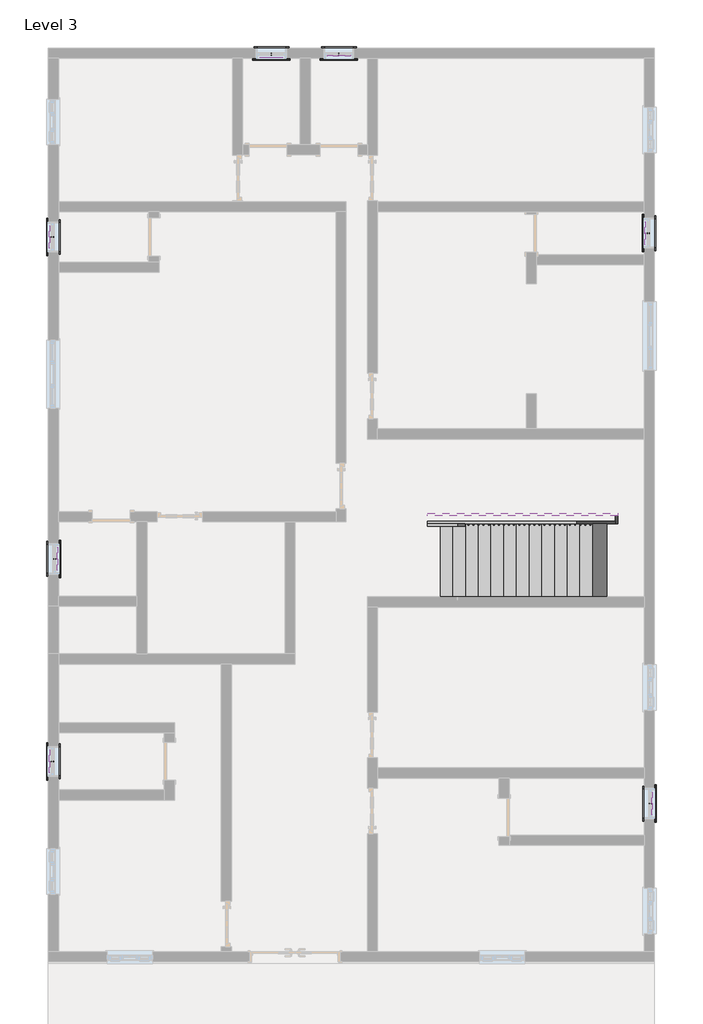
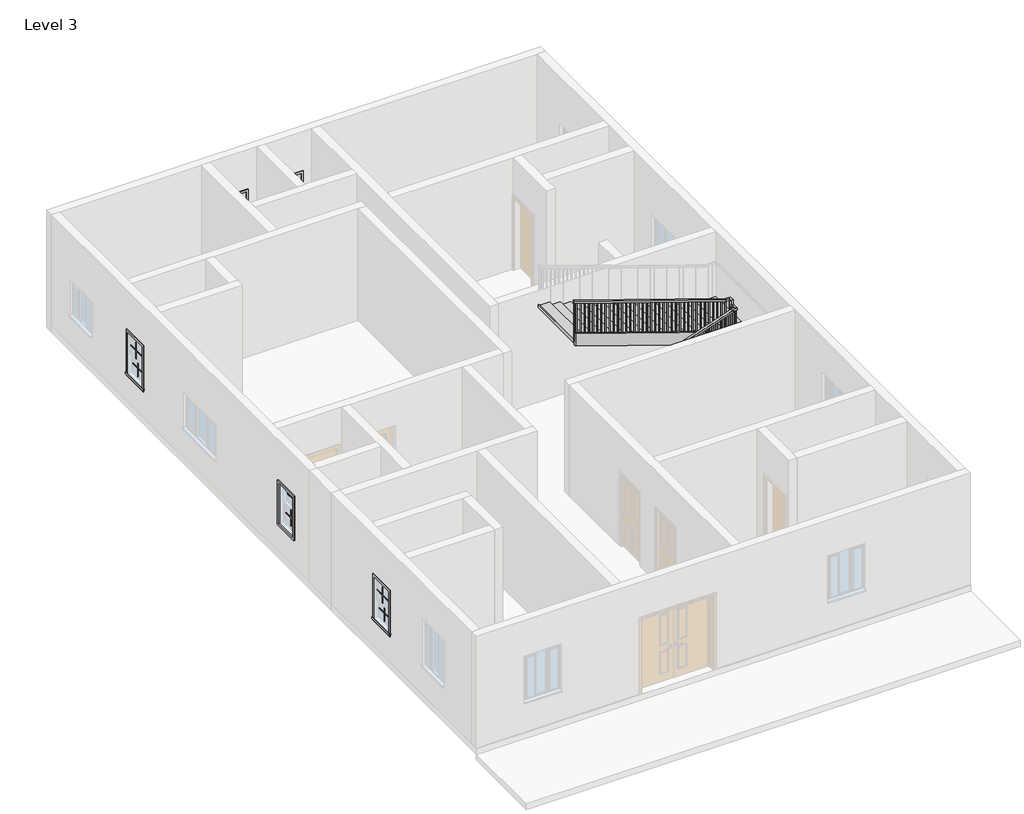
# One storey, part 3 of 3: 28 proxies, 6 members, 1 railing, 1 stair flight.
"""IFC4 building model written with IfcOpenShell, lengths in millimetres."""

from ifc_helpers import new_model, si_unit, frame, origin, place, context, project, spatial, polyline, outline, extrude, faceted_brep, transform, mapped, element, save
from components import muntin_pattern_2x2_muntin_pattern_2x2_eba6c5fb, trim_window_exterior_flat_with_sill_278e6a94, trim_window_interior_flat_picture_frame_e9fd5f45, stair_flight_242bbcd4

model = new_model("IFC4")

# Units and contexts
model_context = context("Model", 3, world=origin())
ifc_project = project(units=[si_unit("LENGTHUNIT", "METRE", prefix="MILLI")], contexts=[model_context])

# Site, building, storey
site = spatial("IfcSite", under=ifc_project)
building = spatial("IfcBuilding", under=site)
storey = spatial("IfcBuildingStorey", under=building, Name="Level 3", Elevation=6096.0)

# Proxies
placement = place(None, origin())
muntin_pattern_2x2_muntin_pattern_2x2_shape = muntin_pattern_2x2_muntin_pattern_2x2_eba6c5fb(model_context)
element("IfcBuildingElementProxy", 1, Name="Muntin Pattern_2x2 : Muntin Pattern_2x2", ObjectType="Muntin Pattern_2x2 : Muntin Pattern_2x2", at=placement, inside=storey, context=model_context, shape_type="MappedRepresentation", body=[
    mapped(muntin_pattern_2x2_muntin_pattern_2x2_shape, transform((-6096.8589448, 5183.1303322, 7566.025), x_axis=(0.0, 1.0, 0.0), y_axis=(-1.0, 0.0, 0.0), z_axis=(0.0, 0.0, 1.0))),
])
element("IfcBuildingElementProxy", 2, Name="Muntin Pattern_2x2 : Muntin Pattern_2x2", ObjectType="Muntin Pattern_2x2 : Muntin Pattern_2x2", at=placement, inside=storey, context=model_context, shape_type="MappedRepresentation", body=[
    mapped(muntin_pattern_2x2_muntin_pattern_2x2_shape, transform((-6052.4089448, 5183.1303322, 7086.6), x_axis=(0.0, 1.0, 0.0), y_axis=(-1.0, 0.0, 0.0), z_axis=(0.0, 0.0, 1.0))),
])
element("IfcBuildingElementProxy", 3, Name="Muntin Pattern_2x2 : Muntin Pattern_2x2", ObjectType="Muntin Pattern_2x2 : Muntin Pattern_2x2", at=placement, inside=storey, context=model_context, shape_type="MappedRepresentation", body=[
    mapped(muntin_pattern_2x2_muntin_pattern_2x2_shape, transform((-1673.5309118, 8787.5224079, 7566.025), x_axis=(-1.0, 0.0, 0.0), y_axis=(0.0, -1.0, 0.0), z_axis=(0.0, 0.0, 1.0))),
])
element("IfcBuildingElementProxy", 4, Name="Muntin Pattern_2x2 : Muntin Pattern_2x2", ObjectType="Muntin Pattern_2x2 : Muntin Pattern_2x2", at=placement, inside=storey, context=model_context, shape_type="MappedRepresentation", body=[
    mapped(muntin_pattern_2x2_muntin_pattern_2x2_shape, transform((-1673.5309118, 8831.9724079, 7086.6), x_axis=(-1.0, 0.0, 0.0), y_axis=(0.0, -1.0, 0.0), z_axis=(0.0, 0.0, 1.0))),
])
element("IfcBuildingElementProxy", 5, Name="Muntin Pattern_2x2 : Muntin Pattern_2x2", ObjectType="Muntin Pattern_2x2 : Muntin Pattern_2x2", at=placement, inside=storey, context=model_context, shape_type="MappedRepresentation", body=[
    mapped(muntin_pattern_2x2_muntin_pattern_2x2_shape, transform((-324.5451949, 8787.5224079, 7566.025), x_axis=(-1.0, 0.0, 0.0), y_axis=(0.0, -1.0, 0.0), z_axis=(0.0, 0.0, 1.0))),
])
element("IfcBuildingElementProxy", 6, Name="Muntin Pattern_2x2 : Muntin Pattern_2x2", ObjectType="Muntin Pattern_2x2 : Muntin Pattern_2x2", at=placement, inside=storey, context=model_context, shape_type="MappedRepresentation", body=[
    mapped(muntin_pattern_2x2_muntin_pattern_2x2_shape, transform((-324.5451949, 8831.9724079, 7086.6), x_axis=(-1.0, 0.0, 0.0), y_axis=(0.0, -1.0, 0.0), z_axis=(0.0, 0.0, 1.0))),
])
element("IfcBuildingElementProxy", 7, Name="Muntin Pattern_2x2 : Muntin Pattern_2x2", ObjectType="Muntin Pattern_2x2 : Muntin Pattern_2x2", at=placement, inside=storey, context=model_context, shape_type="MappedRepresentation", body=[
    mapped(muntin_pattern_2x2_muntin_pattern_2x2_shape, transform((5813.4689795, 5259.3303322, 7566.025), x_axis=(0.0, 1.0, 0.0), y_axis=(-1.0, 0.0, 0.0), z_axis=(0.0, 0.0, 1.0))),
])
element("IfcBuildingElementProxy", 8, Name="Muntin Pattern_2x2 : Muntin Pattern_2x2", ObjectType="Muntin Pattern_2x2 : Muntin Pattern_2x2", at=placement, inside=storey, context=model_context, shape_type="MappedRepresentation", body=[
    mapped(muntin_pattern_2x2_muntin_pattern_2x2_shape, transform((5857.9189795, 5259.3303322, 7086.6), x_axis=(0.0, 1.0, 0.0), y_axis=(-1.0, 0.0, 0.0), z_axis=(0.0, 0.0, 1.0))),
])
element("IfcBuildingElementProxy", 9, Name="Muntin Pattern_2x2 : Muntin Pattern_2x2", ObjectType="Muntin Pattern_2x2 : Muntin Pattern_2x2", at=placement, inside=storey, context=model_context, shape_type="MappedRepresentation", body=[
    mapped(muntin_pattern_2x2_muntin_pattern_2x2_shape, transform((5946.8189795, -6133.2488489, 7566.025), x_axis=(0.0, -1.0, 0.0), y_axis=(1.0, 0.0, 0.0), z_axis=(0.0, 0.0, 1.0))),
])
element("IfcBuildingElementProxy", 10, Name="Muntin Pattern_2x2 : Muntin Pattern_2x2", ObjectType="Muntin Pattern_2x2 : Muntin Pattern_2x2", at=placement, inside=storey, context=model_context, shape_type="MappedRepresentation", body=[
    mapped(muntin_pattern_2x2_muntin_pattern_2x2_shape, transform((5902.3689795, -6133.2488489, 7086.6), x_axis=(0.0, -1.0, 0.0), y_axis=(1.0, 0.0, 0.0), z_axis=(0.0, 0.0, 1.0))),
])
element("IfcBuildingElementProxy", 11, Name="Muntin Pattern_2x2 : Muntin Pattern_2x2", ObjectType="Muntin Pattern_2x2 : Muntin Pattern_2x2", at=placement, inside=storey, context=model_context, shape_type="MappedRepresentation", body=[
    mapped(muntin_pattern_2x2_muntin_pattern_2x2_shape, transform((-6096.8589448, -5291.0659014, 7566.025), x_axis=(0.0, 1.0, 0.0), y_axis=(-1.0, 0.0, 0.0), z_axis=(0.0, 0.0, 1.0))),
])
element("IfcBuildingElementProxy", 12, Name="Muntin Pattern_2x2 : Muntin Pattern_2x2", ObjectType="Muntin Pattern_2x2 : Muntin Pattern_2x2", at=placement, inside=storey, context=model_context, shape_type="MappedRepresentation", body=[
    mapped(muntin_pattern_2x2_muntin_pattern_2x2_shape, transform((-6052.4089448, -5291.0659014, 7086.6), x_axis=(0.0, 1.0, 0.0), y_axis=(-1.0, 0.0, 0.0), z_axis=(0.0, 0.0, 1.0))),
])
element("IfcBuildingElementProxy", 13, Name="Muntin Pattern_2x2 : Muntin Pattern_2x2", ObjectType="Muntin Pattern_2x2 : Muntin Pattern_2x2", at=placement, inside=storey, context=model_context, shape_type="MappedRepresentation", body=[
    mapped(muntin_pattern_2x2_muntin_pattern_2x2_shape, transform((-5963.5089448, -1246.1159014, 7566.025), x_axis=(0.0, -1.0, 0.0), y_axis=(1.0, 0.0, 0.0), z_axis=(0.0, 0.0, 1.0))),
])
element("IfcBuildingElementProxy", 14, Name="Muntin Pattern_2x2 : Muntin Pattern_2x2", ObjectType="Muntin Pattern_2x2 : Muntin Pattern_2x2", at=placement, inside=storey, context=model_context, shape_type="MappedRepresentation", body=[
    mapped(muntin_pattern_2x2_muntin_pattern_2x2_shape, transform((-6007.9589448, -1246.1159014, 7086.6), x_axis=(0.0, -1.0, 0.0), y_axis=(1.0, 0.0, 0.0), z_axis=(0.0, 0.0, 1.0))),
])
trim_window_exterior_flat_with_sill_shape = trim_window_exterior_flat_with_sill_278e6a94(model_context)
element("IfcBuildingElementProxy", 15, Name="Trim-Window-Exterior-Flat : with Sill", ObjectType="Trim-Window-Exterior-Flat : with Sill", at=placement, inside=storey, context=model_context, shape_type="MappedRepresentation", body=[
    mapped(trim_window_exterior_flat_with_sill_shape, transform((-6131.7839448, 5183.1303322, 8077.2), x_axis=(0.0, -1.0, 0.0), y_axis=(0.0, 0.0, 1.0), z_axis=(-1.0, 0.0, 0.0))),
])
element("IfcBuildingElementProxy", 16, Name="Trim-Window-Exterior-Flat : with Sill", ObjectType="Trim-Window-Exterior-Flat : with Sill", at=placement, inside=storey, context=model_context, shape_type="MappedRepresentation", body=[
    mapped(trim_window_exterior_flat_with_sill_shape, transform((-1673.5309118, 8752.5974079, 8077.2), x_axis=(1.0, 0.0, 0.0), y_axis=(0.0, 0.0, 1.0), z_axis=(0.0, -1.0, 0.0))),
])
element("IfcBuildingElementProxy", 17, Name="Trim-Window-Exterior-Flat : with Sill", ObjectType="Trim-Window-Exterior-Flat : with Sill", at=placement, inside=storey, context=model_context, shape_type="MappedRepresentation", body=[
    mapped(trim_window_exterior_flat_with_sill_shape, transform((-324.5451949, 8752.5974079, 8077.2), x_axis=(1.0, 0.0, 0.0), y_axis=(0.0, 0.0, 1.0), z_axis=(0.0, -1.0, 0.0))),
])
element("IfcBuildingElementProxy", 18, Name="Trim-Window-Exterior-Flat : with Sill", ObjectType="Trim-Window-Exterior-Flat : with Sill", at=placement, inside=storey, context=model_context, shape_type="MappedRepresentation", body=[
    mapped(trim_window_exterior_flat_with_sill_shape, transform((5778.5439795, 5259.3303322, 8077.2), x_axis=(0.0, -1.0, 0.0), y_axis=(0.0, 0.0, 1.0), z_axis=(-1.0, 0.0, 0.0))),
])
element("IfcBuildingElementProxy", 19, Name="Trim-Window-Exterior-Flat : with Sill", ObjectType="Trim-Window-Exterior-Flat : with Sill", at=placement, inside=storey, context=model_context, shape_type="MappedRepresentation", body=[
    mapped(trim_window_exterior_flat_with_sill_shape, transform((5981.7439795, -6133.2488489, 8077.2), x_axis=(0.0, 1.0, 0.0), y_axis=(0.0, 0.0, 1.0), z_axis=(1.0, 0.0, 0.0))),
])
element("IfcBuildingElementProxy", 20, Name="Trim-Window-Exterior-Flat : with Sill", ObjectType="Trim-Window-Exterior-Flat : with Sill", at=placement, inside=storey, context=model_context, shape_type="MappedRepresentation", body=[
    mapped(trim_window_exterior_flat_with_sill_shape, transform((-6131.7839448, -5291.0659014, 8077.2), x_axis=(0.0, -1.0, 0.0), y_axis=(0.0, 0.0, 1.0), z_axis=(-1.0, 0.0, 0.0))),
])
element("IfcBuildingElementProxy", 21, Name="Trim-Window-Exterior-Flat : with Sill", ObjectType="Trim-Window-Exterior-Flat : with Sill", at=placement, inside=storey, context=model_context, shape_type="MappedRepresentation", body=[
    mapped(trim_window_exterior_flat_with_sill_shape, transform((-5928.5839448, -1246.1159014, 8077.2), x_axis=(0.0, 1.0, 0.0), y_axis=(0.0, 0.0, 1.0), z_axis=(1.0, 0.0, 0.0))),
])
trim_window_interior_flat_picture_frame_shape = trim_window_interior_flat_picture_frame_e9fd5f45(model_context)
element("IfcBuildingElementProxy", 22, Name="Trim-Window-Interior-Flat : Picture Frame", ObjectType="Trim-Window-Interior-Flat : Picture Frame", at=placement, inside=storey, context=model_context, shape_type="MappedRepresentation", body=[
    mapped(trim_window_interior_flat_picture_frame_shape, transform((-5928.5839448, 5183.1303322, 8077.2), x_axis=(0.0, 1.0, 0.0), y_axis=(0.0, 0.0, 1.0), z_axis=(1.0, 0.0, 0.0))),
])
element("IfcBuildingElementProxy", 23, Name="Trim-Window-Interior-Flat : Picture Frame", ObjectType="Trim-Window-Interior-Flat : Picture Frame", at=placement, inside=storey, context=model_context, shape_type="MappedRepresentation", body=[
    mapped(trim_window_interior_flat_picture_frame_shape, transform((-1673.5309118, 8955.7974079, 8077.2), x_axis=(-1.0, 0.0, 0.0), y_axis=(0.0, 0.0, 1.0), z_axis=(0.0, 1.0, 0.0))),
])
element("IfcBuildingElementProxy", 24, Name="Trim-Window-Interior-Flat : Picture Frame", ObjectType="Trim-Window-Interior-Flat : Picture Frame", at=placement, inside=storey, context=model_context, shape_type="MappedRepresentation", body=[
    mapped(trim_window_interior_flat_picture_frame_shape, transform((-324.5451949, 8955.7974079, 8077.2), x_axis=(-1.0, 0.0, 0.0), y_axis=(0.0, 0.0, 1.0), z_axis=(0.0, 1.0, 0.0))),
])
element("IfcBuildingElementProxy", 25, Name="Trim-Window-Interior-Flat : Picture Frame", ObjectType="Trim-Window-Interior-Flat : Picture Frame", at=placement, inside=storey, context=model_context, shape_type="MappedRepresentation", body=[
    mapped(trim_window_interior_flat_picture_frame_shape, transform((5981.7439795, 5259.3303322, 8077.2), x_axis=(0.0, 1.0, 0.0), y_axis=(0.0, 0.0, 1.0), z_axis=(1.0, 0.0, 0.0))),
])
element("IfcBuildingElementProxy", 26, Name="Trim-Window-Interior-Flat : Picture Frame", ObjectType="Trim-Window-Interior-Flat : Picture Frame", at=placement, inside=storey, context=model_context, shape_type="MappedRepresentation", body=[
    mapped(trim_window_interior_flat_picture_frame_shape, transform((5778.5439795, -6133.2488489, 8077.2), x_axis=(0.0, -1.0, 0.0), y_axis=(0.0, 0.0, 1.0), z_axis=(-1.0, 0.0, 0.0))),
])
element("IfcBuildingElementProxy", 27, Name="Trim-Window-Interior-Flat : Picture Frame", ObjectType="Trim-Window-Interior-Flat : Picture Frame", at=placement, inside=storey, context=model_context, shape_type="MappedRepresentation", body=[
    mapped(trim_window_interior_flat_picture_frame_shape, transform((-5928.5839448, -5291.0659014, 8077.2), x_axis=(0.0, 1.0, 0.0), y_axis=(0.0, 0.0, 1.0), z_axis=(1.0, 0.0, 0.0))),
])
element("IfcBuildingElementProxy", 28, Name="Trim-Window-Interior-Flat : Picture Frame", ObjectType="Trim-Window-Interior-Flat : Picture Frame", at=placement, inside=storey, context=model_context, shape_type="MappedRepresentation", body=[
    mapped(trim_window_interior_flat_picture_frame_shape, transform((-6131.7839448, -1246.1159014, 8077.2), x_axis=(0.0, -1.0, 0.0), y_axis=(0.0, 0.0, 1.0), z_axis=(-1.0, 0.0, 0.0))),
])

# Members
element("IfcMember", 29, ObjectType="Stringer - 2\" Width", at=placement, inside=storey, context=model_context, shape_type="SweptSolid", body=[
    extrude(outline(polyline([(6289.7751932, 1449.3932247), (6096.0, 1449.3932247), (6096.0, 1827.5890963), (7236.094539, 5195.8669505), (7543.8, 5195.8669505), (7543.8, 5154.2649181), (6289.7751932, 1449.3932247)])), frame((0.0, -541.2659014, 0.0), z_axis=(0.0, 1.0, 0.0), x_axis=(0.0, 0.0, 1.0)), (0.0, 0.0, 1.0), 50.8),
])
element("IfcMember", 30, ObjectType="Stringer - 2\" Width", at=placement, inside=storey, context=model_context, shape_type="SweptSolid", body=[
    extrude(outline(polyline([(5246.6669505, -541.2659014), (5195.8669505, -541.2659014), (5195.8669505, -388.7910016), (5246.6669505, -388.7910016), (5246.6669505, -541.2659014)])), frame((0.0, 0.0, 7239.0), z_axis=(0.0, 0.0, 1.0), x_axis=(1.0, 0.0, 0.0)), (0.0, 0.0, 1.0), 304.8),
])
element("IfcMember", 31, ObjectType="Stringer - 2\" Width", at=placement, inside=storey, context=model_context, shape_type="SweptSolid", body=[
    extrude(outline(polyline([(7339.0143208, 5246.6669505), (7660.8012358, 5246.6669505), (8946.1022784, 1449.3932247), (8624.3153634, 1449.3932247), (7339.0143208, 5246.6669505)])), frame((0.0, -388.7910016, 0.0), z_axis=(0.0, 1.0, 0.0), x_axis=(0.0, 0.0, 1.0)), (0.0, 0.0, 1.0), 50.8),
])
element("IfcMember", 32, ObjectType="Stringer - 2\" Width", at=placement, inside=storey, context=model_context, shape_type="SweptSolid", body=[
    extrude(outline(polyline([(6289.7751932, 1449.3932247), (6096.0, 1449.3932247), (6096.0, 1827.5890963), (7448.1142723, 5822.2548051), (7543.8, 5822.2548051), (7543.8, 5154.2649181), (6289.7751932, 1449.3932247)])), frame((0.0, -2116.0659014, 0.0), z_axis=(0.0, 1.0, 0.0), x_axis=(0.0, 0.0, 1.0)), (0.0, 0.0, 1.0), 50.8),
])
element("IfcMember", 33, ObjectType="Stringer - 2\" Width", at=placement, inside=storey, context=model_context, shape_type="SweptSolid", body=[
    extrude(outline(polyline([(5873.0548051, -2116.0659014), (5822.2548051, -2116.0659014), (5822.2548051, 1185.9340986), (5873.0548051, 1185.9340986), (5873.0548051, -2116.0659014)])), frame((0.0, 0.0, 7239.0), z_axis=(0.0, 0.0, 1.0), x_axis=(1.0, 0.0, 0.0)), (0.0, 0.0, 1.0), 304.8),
])
element("IfcMember", 34, ObjectType="Stringer - 2\" Width", at=placement, inside=storey, context=model_context, shape_type="SweptSolid", body=[
    extrude(outline(polyline([(7239.0, 5873.0548051), (7448.7815025, 5873.0548051), (8946.1022784, 1449.3932247), (8624.3153634, 1449.3932247), (7239.0, 5542.1477288), (7239.0, 5873.0548051)])), frame((0.0, 1185.9340986, 0.0), z_axis=(0.0, 1.0, 0.0), x_axis=(0.0, 0.0, 1.0)), (0.0, 0.0, 1.0), 50.8),
])

# Railing
element("IfcRailing", 35, ObjectType="Handrail - Rectangular", at=placement, inside=storey, context=model_context, shape_type="SolidModel", body=[
    faceted_brep([(1449.3932247, -541.2659014, 7096.125), (1449.3932247, -541.2659014, 7042.4913852), (1449.3932247, -592.0659014, 7042.4913852), (1449.3932247, -592.0659014, 7096.125), (5170.4669505, -541.2659014, 8356.1963098), (5221.2669505, -541.2659014, 8319.7651551), (5221.2669505, -592.0659014, 8319.7651551), (5170.4669505, -592.0659014, 8356.1963098), (5170.4669505, -541.2659014, 8382.0), (5221.2669505, -541.2659014, 8331.2), (5221.2669505, -592.0659014, 8331.2), (5170.4669505, -592.0659014, 8382.0), (5246.6669505, -541.2659014, 8382.0), (5246.6669505, -541.2659014, 8331.2), (5297.4669505, -592.0659014, 8331.2), (5297.4669505, -592.0659014, 8382.0), (5246.6669505, -465.0659014, 8382.0), (5246.6669505, -465.0659014, 8331.2), (5297.4669505, -465.0659014, 8331.2), (5297.4669505, -465.0659014, 8382.0), (5246.6669505, -414.1910016, 8382.0), (5246.6669505, -363.3910016, 8331.2), (5297.4669505, -363.3910016, 8331.2), (5297.4669505, -414.1910016, 8382.0), (5246.6669505, -414.1910016, 8493.5286902), (5246.6669505, -363.3910016, 8442.7286902), (5297.4669505, -363.3910016, 8442.7286902), (5297.4669505, -414.1910016, 8493.5286902), (5246.6669505, -337.9910016, 8493.5286902), (5246.6669505, -337.9910016, 8442.7286902), (5297.4669505, -287.1910016, 8442.7286902), (5297.4669505, -287.1910016, 8493.5286902), (5170.4669505, -337.9910016, 8493.5286902), (5162.099099, -337.9910016, 8442.7286902), (5162.099099, -287.1910016, 8442.7286902), (5170.4669505, -287.1910016, 8493.5286902), (1449.3932247, -337.9910016, 9753.6), (1449.3932247, -287.1910016, 9753.6), (1449.3932247, -287.1910016, 9699.9663852), (1449.3932247, -337.9910016, 9699.9663852)], [[[0, 1, 2, 3]], [[1, 0, 4, 5]], [[2, 1, 5, 6]], [[3, 2, 6, 7]], [[0, 3, 7, 4]], [[5, 4, 8, 9]], [[6, 5, 9, 10]], [[7, 6, 10, 11]], [[4, 7, 11, 8]], [[9, 8, 12, 13]], [[10, 9, 13, 14]], [[11, 10, 14, 15]], [[8, 11, 15, 12]], [[13, 12, 16, 17]], [[14, 13, 17, 18]], [[15, 14, 18, 19]], [[12, 15, 19, 16]], [[17, 16, 20, 21]], [[18, 17, 21, 22]], [[19, 18, 22, 23]], [[16, 19, 23, 20]], [[21, 20, 24, 25]], [[22, 21, 25, 26]], [[23, 22, 26, 27]], [[20, 23, 27, 24]], [[25, 24, 28, 29]], [[26, 25, 29, 30]], [[27, 26, 30, 31]], [[24, 27, 31, 28]], [[29, 28, 32, 33]], [[30, 29, 33, 34]], [[31, 30, 34, 35]], [[28, 31, 35, 32]], [[36, 37, 38, 39]], [[33, 32, 36, 39]], [[34, 33, 39, 38]], [[35, 34, 38, 37]], [[32, 35, 37, 36]]]),
    extrude(outline(polyline([(9681.6976686, 1503.3419505), (8753.475, 1503.3419505), (8753.475, 1522.3919505), (9675.246746, 1522.3919505), (9681.6976686, 1503.3419505)])), frame((0.0, -322.1160016, 0.0), z_axis=(0.0, 1.0, 0.0), x_axis=(0.0, 0.0, 1.0)), (0.0, 0.0, 1.0), 19.05),
    extrude(outline(polyline([(9647.2927482, 1604.9419505), (8753.475, 1604.9419505), (8753.475, 1623.9919505), (9640.8418257, 1623.9919505), (9647.2927482, 1604.9419505)])), frame((0.0, -322.1160016, 0.0), z_axis=(0.0, 1.0, 0.0), x_axis=(0.0, 0.0, 1.0)), (0.0, 0.0, 1.0), 19.05),
    extrude(outline(polyline([(9612.8878279, 1706.5419505), (8667.75, 1706.5419505), (8667.75, 1725.5919505), (9606.4369054, 1725.5919505), (9612.8878279, 1706.5419505)])), frame((0.0, -322.1160016, 0.0), z_axis=(0.0, 1.0, 0.0), x_axis=(0.0, 0.0, 1.0)), (0.0, 0.0, 1.0), 19.05),
    extrude(outline(polyline([(9578.4829076, 1808.1419505), (8667.75, 1808.1419505), (8667.75, 1827.1919505), (9572.031985, 1827.1919505), (9578.4829076, 1808.1419505)])), frame((0.0, -322.1160016, 0.0), z_axis=(0.0, 1.0, 0.0), x_axis=(0.0, 0.0, 1.0)), (0.0, 0.0, 1.0), 19.05),
    extrude(outline(polyline([(9544.0779873, 1909.7419505), (8667.75, 1909.7419505), (8667.75, 1928.7919505), (9537.6270647, 1928.7919505), (9544.0779873, 1909.7419505)])), frame((0.0, -322.1160016, 0.0), z_axis=(0.0, 1.0, 0.0), x_axis=(0.0, 0.0, 1.0)), (0.0, 0.0, 1.0), 19.05),
    extrude(outline(polyline([(9509.6730669, 2011.3419505), (8582.025, 2011.3419505), (8582.025, 2030.3919505), (9503.2221444, 2030.3919505), (9509.6730669, 2011.3419505)])), frame((0.0, -322.1160016, 0.0), z_axis=(0.0, 1.0, 0.0), x_axis=(0.0, 0.0, 1.0)), (0.0, 0.0, 1.0), 19.05),
    extrude(outline(polyline([(9475.2681466, 2112.9419505), (8582.025, 2112.9419505), (8582.025, 2131.9919505), (9468.817224, 2131.9919505), (9475.2681466, 2112.9419505)])), frame((0.0, -322.1160016, 0.0), z_axis=(0.0, 1.0, 0.0), x_axis=(0.0, 0.0, 1.0)), (0.0, 0.0, 1.0), 19.05),
    extrude(outline(polyline([(9440.8632263, 2214.5419505), (8496.3, 2214.5419505), (8496.3, 2233.5919505), (9434.4123037, 2233.5919505), (9440.8632263, 2214.5419505)])), frame((0.0, -322.1160016, 0.0), z_axis=(0.0, 1.0, 0.0), x_axis=(0.0, 0.0, 1.0)), (0.0, 0.0, 1.0), 19.05),
    extrude(outline(polyline([(9406.4583059, 2316.1419505), (8496.3, 2316.1419505), (8496.3, 2335.1919505), (9400.0073834, 2335.1919505), (9406.4583059, 2316.1419505)])), frame((0.0, -322.1160016, 0.0), z_axis=(0.0, 1.0, 0.0), x_axis=(0.0, 0.0, 1.0)), (0.0, 0.0, 1.0), 19.05),
    extrude(outline(polyline([(9372.0533856, 2417.7419505), (8496.3, 2417.7419505), (8496.3, 2436.7919505), (9365.6024631, 2436.7919505), (9372.0533856, 2417.7419505)])), frame((0.0, -322.1160016, 0.0), z_axis=(0.0, 1.0, 0.0), x_axis=(0.0, 0.0, 1.0)), (0.0, 0.0, 1.0), 19.05),
    extrude(outline(polyline([(9337.6484653, 2519.3419505), (8410.575, 2519.3419505), (8410.575, 2538.3919505), (9331.1975427, 2538.3919505), (9337.6484653, 2519.3419505)])), frame((0.0, -322.1160016, 0.0), z_axis=(0.0, 1.0, 0.0), x_axis=(0.0, 0.0, 1.0)), (0.0, 0.0, 1.0), 19.05),
    extrude(outline(polyline([(9303.243545, 2620.9419505), (8410.575, 2620.9419505), (8410.575, 2639.9919505), (9296.7926224, 2639.9919505), (9303.243545, 2620.9419505)])), frame((0.0, -322.1160016, 0.0), z_axis=(0.0, 1.0, 0.0), x_axis=(0.0, 0.0, 1.0)), (0.0, 0.0, 1.0), 19.05),
    extrude(outline(polyline([(9268.8386246, 2722.5419505), (8324.85, 2722.5419505), (8324.85, 2741.5919505), (9262.3877021, 2741.5919505), (9268.8386246, 2722.5419505)])), frame((0.0, -322.1160016, 0.0), z_axis=(0.0, 1.0, 0.0), x_axis=(0.0, 0.0, 1.0)), (0.0, 0.0, 1.0), 19.05),
    extrude(outline(polyline([(9234.4337043, 2824.1419505), (8324.85, 2824.1419505), (8324.85, 2843.1919505), (9227.9827817, 2843.1919505), (9234.4337043, 2824.1419505)])), frame((0.0, -322.1160016, 0.0), z_axis=(0.0, 1.0, 0.0), x_axis=(0.0, 0.0, 1.0)), (0.0, 0.0, 1.0), 19.05),
    extrude(outline(polyline([(9200.028784, 2925.7419505), (8324.85, 2925.7419505), (8324.85, 2944.7919505), (9193.5778614, 2944.7919505), (9200.028784, 2925.7419505)])), frame((0.0, -322.1160016, 0.0), z_axis=(0.0, 1.0, 0.0), x_axis=(0.0, 0.0, 1.0)), (0.0, 0.0, 1.0), 19.05),
    extrude(outline(polyline([(9165.6238636, 3027.3419505), (8239.125, 3027.3419505), (8239.125, 3046.3919505), (9159.1729411, 3046.3919505), (9165.6238636, 3027.3419505)])), frame((0.0, -322.1160016, 0.0), z_axis=(0.0, 1.0, 0.0), x_axis=(0.0, 0.0, 1.0)), (0.0, 0.0, 1.0), 19.05),
    extrude(outline(polyline([(9131.2189433, 3128.9419505), (8239.125, 3128.9419505), (8239.125, 3147.9919505), (9124.7680208, 3147.9919505), (9131.2189433, 3128.9419505)])), frame((0.0, -322.1160016, 0.0), z_axis=(0.0, 1.0, 0.0), x_axis=(0.0, 0.0, 1.0)), (0.0, 0.0, 1.0), 19.05),
    extrude(outline(polyline([(9096.814023, 3230.5419505), (8153.4, 3230.5419505), (8153.4, 3249.5919505), (9090.3631004, 3249.5919505), (9096.814023, 3230.5419505)])), frame((0.0, -322.1160016, 0.0), z_axis=(0.0, 1.0, 0.0), x_axis=(0.0, 0.0, 1.0)), (0.0, 0.0, 1.0), 19.05),
    extrude(outline(polyline([(9062.4091027, 3332.1419505), (8153.4, 3332.1419505), (8153.4, 3351.1919505), (9055.9581801, 3351.1919505), (9062.4091027, 3332.1419505)])), frame((0.0, -322.1160016, 0.0), z_axis=(0.0, 1.0, 0.0), x_axis=(0.0, 0.0, 1.0)), (0.0, 0.0, 1.0), 19.05),
    extrude(outline(polyline([(9028.0041823, 3433.7419505), (8153.4, 3433.7419505), (8153.4, 3452.7919505), (9021.5532598, 3452.7919505), (9028.0041823, 3433.7419505)])), frame((0.0, -322.1160016, 0.0), z_axis=(0.0, 1.0, 0.0), x_axis=(0.0, 0.0, 1.0)), (0.0, 0.0, 1.0), 19.05),
    extrude(outline(polyline([(8993.599262, 3535.3419505), (8067.675, 3535.3419505), (8067.675, 3554.3919505), (8987.1483394, 3554.3919505), (8993.599262, 3535.3419505)])), frame((0.0, -322.1160016, 0.0), z_axis=(0.0, 1.0, 0.0), x_axis=(0.0, 0.0, 1.0)), (0.0, 0.0, 1.0), 19.05),
    extrude(outline(polyline([(8959.1943417, 3636.9419505), (8067.675, 3636.9419505), (8067.675, 3655.9919505), (8952.7434191, 3655.9919505), (8959.1943417, 3636.9419505)])), frame((0.0, -322.1160016, 0.0), z_axis=(0.0, 1.0, 0.0), x_axis=(0.0, 0.0, 1.0)), (0.0, 0.0, 1.0), 19.05),
    extrude(outline(polyline([(8924.7894213, 3738.5419505), (7981.95, 3738.5419505), (7981.95, 3757.5919505), (8918.3384988, 3757.5919505), (8924.7894213, 3738.5419505)])), frame((0.0, -322.1160016, 0.0), z_axis=(0.0, 1.0, 0.0), x_axis=(0.0, 0.0, 1.0)), (0.0, 0.0, 1.0), 19.05),
    extrude(outline(polyline([(8890.384501, 3840.1419505), (7981.95, 3840.1419505), (7981.95, 3859.1919505), (8883.9335784, 3859.1919505), (8890.384501, 3840.1419505)])), frame((0.0, -322.1160016, 0.0), z_axis=(0.0, 1.0, 0.0), x_axis=(0.0, 0.0, 1.0)), (0.0, 0.0, 1.0), 19.05),
    extrude(outline(polyline([(8855.9795807, 3941.7419505), (7981.95, 3941.7419505), (7981.95, 3960.7919505), (8849.5286581, 3960.7919505), (8855.9795807, 3941.7419505)])), frame((0.0, -322.1160016, 0.0), z_axis=(0.0, 1.0, 0.0), x_axis=(0.0, 0.0, 1.0)), (0.0, 0.0, 1.0), 19.05),
    extrude(outline(polyline([(8821.5746604, 4043.3419505), (7896.225, 4043.3419505), (7896.225, 4062.3919505), (8815.1237378, 4062.3919505), (8821.5746604, 4043.3419505)])), frame((0.0, -322.1160016, 0.0), z_axis=(0.0, 1.0, 0.0), x_axis=(0.0, 0.0, 1.0)), (0.0, 0.0, 1.0), 19.05),
    extrude(outline(polyline([(8787.16974, 4144.9419505), (7896.225, 4144.9419505), (7896.225, 4163.9919505), (8780.7188175, 4163.9919505), (8787.16974, 4144.9419505)])), frame((0.0, -322.1160016, 0.0), z_axis=(0.0, 1.0, 0.0), x_axis=(0.0, 0.0, 1.0)), (0.0, 0.0, 1.0), 19.05),
    extrude(outline(polyline([(8752.7648197, 4246.5419505), (7810.5, 4246.5419505), (7810.5, 4265.5919505), (8746.3138971, 4265.5919505), (8752.7648197, 4246.5419505)])), frame((0.0, -322.1160016, 0.0), z_axis=(0.0, 1.0, 0.0), x_axis=(0.0, 0.0, 1.0)), (0.0, 0.0, 1.0), 19.05),
    extrude(outline(polyline([(8718.3598994, 4348.1419505), (7810.5, 4348.1419505), (7810.5, 4367.1919505), (8711.9089768, 4367.1919505), (8718.3598994, 4348.1419505)])), frame((0.0, -322.1160016, 0.0), z_axis=(0.0, 1.0, 0.0), x_axis=(0.0, 0.0, 1.0)), (0.0, 0.0, 1.0), 19.05),
    extrude(outline(polyline([(8683.954979, 4449.7419505), (7810.5, 4449.7419505), (7810.5, 4468.7919505), (8677.5040565, 4468.7919505), (8683.954979, 4449.7419505)])), frame((0.0, -322.1160016, 0.0), z_axis=(0.0, 1.0, 0.0), x_axis=(0.0, 0.0, 1.0)), (0.0, 0.0, 1.0), 19.05),
    extrude(outline(polyline([(8649.5500587, 4551.3419505), (7724.775, 4551.3419505), (7724.775, 4570.3919505), (8643.0991361, 4570.3919505), (8649.5500587, 4551.3419505)])), frame((0.0, -322.1160016, 0.0), z_axis=(0.0, 1.0, 0.0), x_axis=(0.0, 0.0, 1.0)), (0.0, 0.0, 1.0), 19.05),
    extrude(outline(polyline([(8615.1451384, 4652.9419505), (7724.775, 4652.9419505), (7724.775, 4671.9919505), (8608.6942158, 4671.9919505), (8615.1451384, 4652.9419505)])), frame((0.0, -322.1160016, 0.0), z_axis=(0.0, 1.0, 0.0), x_axis=(0.0, 0.0, 1.0)), (0.0, 0.0, 1.0), 19.05),
    extrude(outline(polyline([(8580.7402181, 4754.5419505), (7639.05, 4754.5419505), (7639.05, 4773.5919505), (8574.2892955, 4773.5919505), (8580.7402181, 4754.5419505)])), frame((0.0, -322.1160016, 0.0), z_axis=(0.0, 1.0, 0.0), x_axis=(0.0, 0.0, 1.0)), (0.0, 0.0, 1.0), 19.05),
    extrude(outline(polyline([(8546.3352977, 4856.1419505), (7639.05, 4856.1419505), (7639.05, 4875.1919505), (8539.8843752, 4875.1919505), (8546.3352977, 4856.1419505)])), frame((0.0, -322.1160016, 0.0), z_axis=(0.0, 1.0, 0.0), x_axis=(0.0, 0.0, 1.0)), (0.0, 0.0, 1.0), 19.05),
    extrude(outline(polyline([(8511.9303774, 4957.7419505), (7639.05, 4957.7419505), (7639.05, 4976.7919505), (8505.4794548, 4976.7919505), (8511.9303774, 4957.7419505)])), frame((0.0, -322.1160016, 0.0), z_axis=(0.0, 1.0, 0.0), x_axis=(0.0, 0.0, 1.0)), (0.0, 0.0, 1.0), 19.05),
    extrude(outline(polyline([(8477.5254571, 5059.3419505), (7553.325, 5059.3419505), (7553.325, 5078.3919505), (8471.0745345, 5078.3919505), (8477.5254571, 5059.3419505)])), frame((0.0, -322.1160016, 0.0), z_axis=(0.0, 1.0, 0.0), x_axis=(0.0, 0.0, 1.0)), (0.0, 0.0, 1.0), 19.05),
    extrude(outline(polyline([(8443.1205367, 5160.9419505), (7553.325, 5160.9419505), (7553.325, 5179.9919505), (8436.6696142, 5179.9919505), (8443.1205367, 5160.9419505)])), frame((0.0, -322.1160016, 0.0), z_axis=(0.0, 1.0, 0.0), x_axis=(0.0, 0.0, 1.0)), (0.0, 0.0, 1.0), 19.05),
    extrude(outline(polyline([(5262.5419505, -372.9909014), (5262.5419505, -353.9409014), (5281.5919505, -353.9409014), (5281.5919505, -372.9909014), (5262.5419505, -372.9909014)])), frame((0.0, 0.0, 7467.6), z_axis=(0.0, 0.0, 1.0), x_axis=(1.0, 0.0, 0.0)), (0.0, 0.0, 1.0), 975.1286902),
    extrude(outline(polyline([(5262.5419505, -474.5909014), (5262.5419505, -455.5409014), (5281.5919505, -455.5409014), (5281.5919505, -474.5909014), (5262.5419505, -474.5909014)])), frame((0.0, 0.0, 7467.6), z_axis=(0.0, 0.0, 1.0), x_axis=(1.0, 0.0, 0.0)), (0.0, 0.0, 1.0), 863.6),
    extrude(outline(polyline([(5199.0682247, -557.1409014), (5218.1182247, -557.1409014), (5218.1182247, -576.1909014), (5199.0682247, -576.1909014), (5199.0682247, -557.1409014)])), frame((0.0, 0.0, 7381.875), z_axis=(0.0, 0.0, 1.0), x_axis=(1.0, 0.0, 0.0)), (0.0, 0.0, 1.0), 949.325),
    extrude(outline(polyline([(8277.8430558, 5097.4682247), (7381.875, 5097.4682247), (7381.875, 5116.5182247), (8284.2939783, 5116.5182247), (8277.8430558, 5097.4682247)])), frame((0.0, -576.1909014, 0.0), z_axis=(0.0, 1.0, 0.0), x_axis=(0.0, 0.0, 1.0)), (0.0, 0.0, 1.0), 19.05),
    extrude(outline(polyline([(8243.4381354, 4995.8682247), (7381.875, 4995.8682247), (7381.875, 5014.9182247), (8249.889058, 5014.9182247), (8243.4381354, 4995.8682247)])), frame((0.0, -576.1909014, 0.0), z_axis=(0.0, 1.0, 0.0), x_axis=(0.0, 0.0, 1.0)), (0.0, 0.0, 1.0), 19.05),
    extrude(outline(polyline([(8209.0332151, 4894.2682247), (7296.15, 4894.2682247), (7296.15, 4913.3182247), (8215.4841377, 4913.3182247), (8209.0332151, 4894.2682247)])), frame((0.0, -576.1909014, 0.0), z_axis=(0.0, 1.0, 0.0), x_axis=(0.0, 0.0, 1.0)), (0.0, 0.0, 1.0), 19.05),
    extrude(outline(polyline([(8174.6282948, 4792.6682247), (7296.15, 4792.6682247), (7296.15, 4811.7182247), (8181.0792173, 4811.7182247), (8174.6282948, 4792.6682247)])), frame((0.0, -576.1909014, 0.0), z_axis=(0.0, 1.0, 0.0), x_axis=(0.0, 0.0, 1.0)), (0.0, 0.0, 1.0), 19.05),
    extrude(outline(polyline([(8140.2233745, 4691.0682247), (7210.425, 4691.0682247), (7210.425, 4710.1182247), (8146.674297, 4710.1182247), (8140.2233745, 4691.0682247)])), frame((0.0, -576.1909014, 0.0), z_axis=(0.0, 1.0, 0.0), x_axis=(0.0, 0.0, 1.0)), (0.0, 0.0, 1.0), 19.05),
    extrude(outline(polyline([(8105.8184541, 4589.4682247), (7210.425, 4589.4682247), (7210.425, 4608.5182247), (8112.2693767, 4608.5182247), (8105.8184541, 4589.4682247)])), frame((0.0, -576.1909014, 0.0), z_axis=(0.0, 1.0, 0.0), x_axis=(0.0, 0.0, 1.0)), (0.0, 0.0, 1.0), 19.05),
    extrude(outline(polyline([(8071.4135338, 4487.8682247), (7210.425, 4487.8682247), (7210.425, 4506.9182247), (8077.8644564, 4506.9182247), (8071.4135338, 4487.8682247)])), frame((0.0, -576.1909014, 0.0), z_axis=(0.0, 1.0, 0.0), x_axis=(0.0, 0.0, 1.0)), (0.0, 0.0, 1.0), 19.05),
    extrude(outline(polyline([(8037.0086135, 4386.2682247), (7124.7, 4386.2682247), (7124.7, 4405.3182247), (8043.459536, 4405.3182247), (8037.0086135, 4386.2682247)])), frame((0.0, -576.1909014, 0.0), z_axis=(0.0, 1.0, 0.0), x_axis=(0.0, 0.0, 1.0)), (0.0, 0.0, 1.0), 19.05),
    extrude(outline(polyline([(8002.6036931, 4284.6682247), (7124.7, 4284.6682247), (7124.7, 4303.7182247), (8009.0546157, 4303.7182247), (8002.6036931, 4284.6682247)])), frame((0.0, -576.1909014, 0.0), z_axis=(0.0, 1.0, 0.0), x_axis=(0.0, 0.0, 1.0)), (0.0, 0.0, 1.0), 19.05),
    extrude(outline(polyline([(7968.1987728, 4183.0682247), (7038.975, 4183.0682247), (7038.975, 4202.1182247), (7974.6496954, 4202.1182247), (7968.1987728, 4183.0682247)])), frame((0.0, -576.1909014, 0.0), z_axis=(0.0, 1.0, 0.0), x_axis=(0.0, 0.0, 1.0)), (0.0, 0.0, 1.0), 19.05),
    extrude(outline(polyline([(7933.7938525, 4081.4682247), (7038.975, 4081.4682247), (7038.975, 4100.5182247), (7940.244775, 4100.5182247), (7933.7938525, 4081.4682247)])), frame((0.0, -576.1909014, 0.0), z_axis=(0.0, 1.0, 0.0), x_axis=(0.0, 0.0, 1.0)), (0.0, 0.0, 1.0), 19.05),
    extrude(outline(polyline([(7899.3889321, 3979.8682247), (7038.975, 3979.8682247), (7038.975, 3998.9182247), (7905.8398547, 3998.9182247), (7899.3889321, 3979.8682247)])), frame((0.0, -576.1909014, 0.0), z_axis=(0.0, 1.0, 0.0), x_axis=(0.0, 0.0, 1.0)), (0.0, 0.0, 1.0), 19.05),
    extrude(outline(polyline([(7864.9840118, 3878.2682247), (6953.25, 3878.2682247), (6953.25, 3897.3182247), (7871.4349344, 3897.3182247), (7864.9840118, 3878.2682247)])), frame((0.0, -576.1909014, 0.0), z_axis=(0.0, 1.0, 0.0), x_axis=(0.0, 0.0, 1.0)), (0.0, 0.0, 1.0), 19.05),
    extrude(outline(polyline([(7830.5790915, 3776.6682247), (6953.25, 3776.6682247), (6953.25, 3795.7182247), (7837.0300141, 3795.7182247), (7830.5790915, 3776.6682247)])), frame((0.0, -576.1909014, 0.0), z_axis=(0.0, 1.0, 0.0), x_axis=(0.0, 0.0, 1.0)), (0.0, 0.0, 1.0), 19.05),
    extrude(outline(polyline([(7796.1741712, 3675.0682247), (6867.525, 3675.0682247), (6867.525, 3694.1182247), (7802.6250937, 3694.1182247), (7796.1741712, 3675.0682247)])), frame((0.0, -576.1909014, 0.0), z_axis=(0.0, 1.0, 0.0), x_axis=(0.0, 0.0, 1.0)), (0.0, 0.0, 1.0), 19.05),
    extrude(outline(polyline([(7761.7692508, 3573.4682247), (6867.525, 3573.4682247), (6867.525, 3592.5182247), (7768.2201734, 3592.5182247), (7761.7692508, 3573.4682247)])), frame((0.0, -576.1909014, 0.0), z_axis=(0.0, 1.0, 0.0), x_axis=(0.0, 0.0, 1.0)), (0.0, 0.0, 1.0), 19.05),
    extrude(outline(polyline([(7727.3643305, 3471.8682247), (6867.525, 3471.8682247), (6867.525, 3490.9182247), (7733.8152531, 3490.9182247), (7727.3643305, 3471.8682247)])), frame((0.0, -576.1909014, 0.0), z_axis=(0.0, 1.0, 0.0), x_axis=(0.0, 0.0, 1.0)), (0.0, 0.0, 1.0), 19.05),
    extrude(outline(polyline([(7692.9594102, 3370.2682247), (6781.8, 3370.2682247), (6781.8, 3389.3182247), (7699.4103327, 3389.3182247), (7692.9594102, 3370.2682247)])), frame((0.0, -576.1909014, 0.0), z_axis=(0.0, 1.0, 0.0), x_axis=(0.0, 0.0, 1.0)), (0.0, 0.0, 1.0), 19.05),
    extrude(outline(polyline([(7658.5544898, 3268.6682247), (6781.8, 3268.6682247), (6781.8, 3287.7182247), (7665.0054124, 3287.7182247), (7658.5544898, 3268.6682247)])), frame((0.0, -576.1909014, 0.0), z_axis=(0.0, 1.0, 0.0), x_axis=(0.0, 0.0, 1.0)), (0.0, 0.0, 1.0), 19.05),
    extrude(outline(polyline([(7624.1495695, 3167.0682247), (6696.075, 3167.0682247), (6696.075, 3186.1182247), (7630.6004921, 3186.1182247), (7624.1495695, 3167.0682247)])), frame((0.0, -576.1909014, 0.0), z_axis=(0.0, 1.0, 0.0), x_axis=(0.0, 0.0, 1.0)), (0.0, 0.0, 1.0), 19.05),
    extrude(outline(polyline([(7589.7446492, 3065.4682247), (6696.075, 3065.4682247), (6696.075, 3084.5182247), (7596.1955718, 3084.5182247), (7589.7446492, 3065.4682247)])), frame((0.0, -576.1909014, 0.0), z_axis=(0.0, 1.0, 0.0), x_axis=(0.0, 0.0, 1.0)), (0.0, 0.0, 1.0), 19.05),
    extrude(outline(polyline([(7555.3397289, 2963.8682247), (6696.075, 2963.8682247), (6696.075, 2982.9182247), (7561.7906514, 2982.9182247), (7555.3397289, 2963.8682247)])), frame((0.0, -576.1909014, 0.0), z_axis=(0.0, 1.0, 0.0), x_axis=(0.0, 0.0, 1.0)), (0.0, 0.0, 1.0), 19.05),
    extrude(outline(polyline([(7520.9348085, 2862.2682247), (6610.35, 2862.2682247), (6610.35, 2881.3182247), (7527.3857311, 2881.3182247), (7520.9348085, 2862.2682247)])), frame((0.0, -576.1909014, 0.0), z_axis=(0.0, 1.0, 0.0), x_axis=(0.0, 0.0, 1.0)), (0.0, 0.0, 1.0), 19.05),
    extrude(outline(polyline([(7486.5298882, 2760.6682247), (6610.35, 2760.6682247), (6610.35, 2779.7182247), (7492.9808108, 2779.7182247), (7486.5298882, 2760.6682247)])), frame((0.0, -576.1909014, 0.0), z_axis=(0.0, 1.0, 0.0), x_axis=(0.0, 0.0, 1.0)), (0.0, 0.0, 1.0), 19.05),
    extrude(outline(polyline([(7452.1249679, 2659.0682247), (6524.625, 2659.0682247), (6524.625, 2678.1182247), (7458.5758904, 2678.1182247), (7452.1249679, 2659.0682247)])), frame((0.0, -576.1909014, 0.0), z_axis=(0.0, 1.0, 0.0), x_axis=(0.0, 0.0, 1.0)), (0.0, 0.0, 1.0), 19.05),
    extrude(outline(polyline([(7417.7200475, 2557.4682247), (6524.625, 2557.4682247), (6524.625, 2576.5182247), (7424.1709701, 2576.5182247), (7417.7200475, 2557.4682247)])), frame((0.0, -576.1909014, 0.0), z_axis=(0.0, 1.0, 0.0), x_axis=(0.0, 0.0, 1.0)), (0.0, 0.0, 1.0), 19.05),
    extrude(outline(polyline([(7383.3151272, 2455.8682247), (6524.625, 2455.8682247), (6524.625, 2474.9182247), (7389.7660498, 2474.9182247), (7383.3151272, 2455.8682247)])), frame((0.0, -576.1909014, 0.0), z_axis=(0.0, 1.0, 0.0), x_axis=(0.0, 0.0, 1.0)), (0.0, 0.0, 1.0), 19.05),
    extrude(outline(polyline([(7348.9102069, 2354.2682247), (6438.9, 2354.2682247), (6438.9, 2373.3182247), (7355.3611294, 2373.3182247), (7348.9102069, 2354.2682247)])), frame((0.0, -576.1909014, 0.0), z_axis=(0.0, 1.0, 0.0), x_axis=(0.0, 0.0, 1.0)), (0.0, 0.0, 1.0), 19.05),
    extrude(outline(polyline([(7314.5052866, 2252.6682247), (6438.9, 2252.6682247), (6438.9, 2271.7182247), (7320.9562091, 2271.7182247), (7314.5052866, 2252.6682247)])), frame((0.0, -576.1909014, 0.0), z_axis=(0.0, 1.0, 0.0), x_axis=(0.0, 0.0, 1.0)), (0.0, 0.0, 1.0), 19.05),
    extrude(outline(polyline([(7280.1003662, 2151.0682247), (6353.175, 2151.0682247), (6353.175, 2170.1182247), (7286.5512888, 2170.1182247), (7280.1003662, 2151.0682247)])), frame((0.0, -576.1909014, 0.0), z_axis=(0.0, 1.0, 0.0), x_axis=(0.0, 0.0, 1.0)), (0.0, 0.0, 1.0), 19.05),
    extrude(outline(polyline([(7245.6954459, 2049.4682247), (6353.175, 2049.4682247), (6353.175, 2068.5182247), (7252.1463685, 2068.5182247), (7245.6954459, 2049.4682247)])), frame((0.0, -576.1909014, 0.0), z_axis=(0.0, 1.0, 0.0), x_axis=(0.0, 0.0, 1.0)), (0.0, 0.0, 1.0), 19.05),
    extrude(outline(polyline([(7211.2905256, 1947.8682247), (6353.175, 1947.8682247), (6353.175, 1966.9182247), (7217.7414481, 1966.9182247), (7211.2905256, 1947.8682247)])), frame((0.0, -576.1909014, 0.0), z_axis=(0.0, 1.0, 0.0), x_axis=(0.0, 0.0, 1.0)), (0.0, 0.0, 1.0), 19.05),
    extrude(outline(polyline([(7176.8856052, 1846.2682247), (6267.45, 1846.2682247), (6267.45, 1865.3182247), (7183.3365278, 1865.3182247), (7176.8856052, 1846.2682247)])), frame((0.0, -576.1909014, 0.0), z_axis=(0.0, 1.0, 0.0), x_axis=(0.0, 0.0, 1.0)), (0.0, 0.0, 1.0), 19.05),
    extrude(outline(polyline([(7142.4806849, 1744.6682247), (6267.45, 1744.6682247), (6267.45, 1763.7182247), (7148.9316075, 1763.7182247), (7142.4806849, 1744.6682247)])), frame((0.0, -576.1909014, 0.0), z_axis=(0.0, 1.0, 0.0), x_axis=(0.0, 0.0, 1.0)), (0.0, 0.0, 1.0), 19.05),
    extrude(outline(polyline([(7108.0757646, 1643.0682247), (6181.725, 1643.0682247), (6181.725, 1662.1182247), (7114.5266871, 1662.1182247), (7108.0757646, 1643.0682247)])), frame((0.0, -576.1909014, 0.0), z_axis=(0.0, 1.0, 0.0), x_axis=(0.0, 0.0, 1.0)), (0.0, 0.0, 1.0), 19.05),
    extrude(outline(polyline([(7073.6708443, 1541.4682247), (6181.725, 1541.4682247), (6181.725, 1560.5182247), (7080.1217668, 1560.5182247), (7073.6708443, 1541.4682247)])), frame((0.0, -576.1909014, 0.0), z_axis=(0.0, 1.0, 0.0), x_axis=(0.0, 0.0, 1.0)), (0.0, 0.0, 1.0), 19.05),
    extrude(outline(polyline([(5262.5419505, -322.1160016), (5262.5419505, -303.0660016), (5281.5919505, -303.0660016), (5281.5919505, -322.1160016), (5262.5419505, -322.1160016)])), frame((0.0, 0.0, 7467.6), z_axis=(0.0, 0.0, 1.0), x_axis=(1.0, 0.0, 0.0)), (0.0, 0.0, 1.0), 975.1286902),
    extrude(outline(polyline([(5262.5419505, -557.1409014), (5281.5919505, -557.1409014), (5281.5919505, -576.1909014), (5262.5419505, -576.1909014), (5262.5419505, -557.1409014)])), frame((0.0, 0.0, 7467.6), z_axis=(0.0, 0.0, 1.0), x_axis=(1.0, 0.0, 0.0)), (0.0, 0.0, 1.0), 863.6),
    extrude(outline(polyline([(9699.9663852, 1449.3932247), (8753.475, 1449.3932247), (8753.475, 1468.4432247), (9693.5154626, 1468.4432247), (9699.9663852, 1449.3932247)])), frame((0.0, -322.1160016, 0.0), z_axis=(0.0, 1.0, 0.0), x_axis=(0.0, 0.0, 1.0)), (0.0, 0.0, 1.0), 19.05),
    extrude(outline(polyline([(7042.4913852, 1449.3932247), (6181.725, 1449.3932247), (6181.725, 1468.4432247), (7048.9423078, 1468.4432247), (7042.4913852, 1449.3932247)])), frame((0.0, -576.1909014, 0.0), z_axis=(0.0, 1.0, 0.0), x_axis=(0.0, 0.0, 1.0)), (0.0, 0.0, 1.0), 19.05),
])

# Stair flight
stair_flight_shape = stair_flight_242bbcd4(model_context)
element("IfcStairFlight", 36, ObjectType="2\" Tread 1\" Nosing 1/4\" Riser", at=placement, inside=storey, context=model_context, shape_type="MappedRepresentation", body=[
    mapped(stair_flight_shape, transform((0.0, 0.0, 0.0), x_axis=(1.0, 0.0, 0.0), y_axis=(0.0, 1.0, 0.0), z_axis=(0.0, 0.0, 1.0))),
])

save(model, "model.ifc")

# Revit data of these elements
# Type "Muntin Pattern_2x2 : Muntin Pattern_2x2"
#   Width [instance default] = 4' - 0"
#   Thickness = 0' - 0 1/2"
#   Height [instance default] = 4' - 0"
#   Distance = 0' - 0 3/4"
#   Interior Material [instance default] = none
#   Exterior Material [instance default] = none
#   Default Elevation = 0
# Type "Trim-Window-Exterior-Flat : with Sill"
#   Trim Width = 0' - 2 1/4"
#   Trim Thickness_Picture Frame = 0' - 1 1/4"
#   Trim Thickness_with Sill = 0' - 0 3/4"
#   Sill Thickness = 0' - 1 1/4"
#   Opening Width [instance default] = 2' - 0"
#   Opening Height [instance default] = 3' - 0"
#   Default Elevation = 4' - 0"
#   Sill = yes
#   Picture Frame = no
#   Trim Material [instance default] = none
# Type "Trim-Window-Interior-Flat : Picture Frame"
#   Trim Thickness_Picture Frame = 0' - 1 1/4"
#   Trim Width = 0' - 2 1/4"
#   Trim Thickness_with Sill = 0' - 0 3/4"
#   Sill Thickness = 0' - 1 1/4"
#   Opening Width [instance default] = 2' - 0"
#   Opening Height [instance default] = 3' - 0"
#   Default Elevation = 4' - 0"
#   Sill = no
#   Picture Frame = yes
#   Trim Material [instance default] = none
# Type "Handrail - Rectangular"
#   Assembly Code = "C2010400"
#   built-in parameter 1008612 = 0.0416667 (stored number, unit not read)
#   built-in parameter 1008611 = 0.0416667 (stored number, unit not read)
#   built-in parameter 1008609 = 0.333333 (stored number, unit not read)
#   built-in parameter 1008604 = 0.166667 (stored number, unit not read)
#   built-in parameter 1008603 = 0.166667 (stored number, unit not read)
#   Railing Height = 3' - 0"
#   built-in parameter 1008630 = 2
#   built-in parameter 1008610 = 2
#   built-in parameter 1008618 = Baluster - Square : 3/4"
# Elements 1, 2, 3, 4, 5, 6, 7, 8, 9, 10, 11, 12, 13, 14 (IfcBuildingElementProxy, "Muntin Pattern_2x2 : Muntin Pattern_2x2")
#   Width = 1' - 6"
#   Height = 1' - 5 1/8"
#   Interior Material = Wood - Stained
#   Exterior Material = Clad - White
#   Phase Created = New Construction
#   Materials on its faces: "Clad - White", "Wood - Stained"
# Elements 15, 16, 17, 18, 19, 20, 21 (IfcBuildingElementProxy, "Trim-Window-Exterior-Flat : with Sill")
#   Opening Width = 2' - 0"
#   Opening Height = 3' - 6"
#   Trim Material = Clad - White
#   Phase Created = New Construction
#   Materials on its faces: "Clad - White"
# Elements 22, 23, 24, 25, 26, 27, 28 (IfcBuildingElementProxy, "Trim-Window-Interior-Flat : Picture Frame")
#   Opening Width = 2' - 0"
#   Opening Height = 3' - 6"
#   Trim Material = Wood - Stained
#   Phase Created = New Construction
#   Materials on its faces: "Wood - Stained"
# Elements 29, 30, 31, 32, 33, 34 (IfcMember, "Stringer - 2\" Width")
#   Phase Created = New Construction
# Element 35 (IfcRailing, "Handrail - Rectangular")
#   Phase Created = New Construction
# Element 36 (IfcStairFlight, "2\" Tread 1\" Nosing 1/4\" Riser")
#   Phase Created = New Construction
# Materials
#   "Clad - White": class "Wood", colour RGB 242 242 238, transparency 0, Cost = 0
#   "Wood - Stained": class "Wood", colour RGB 224 178 126, transparency 0, Cost = 0
